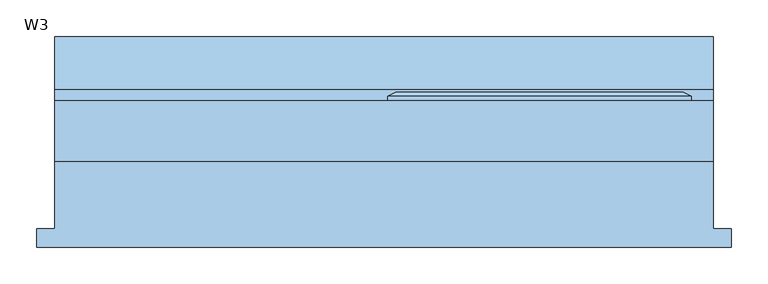
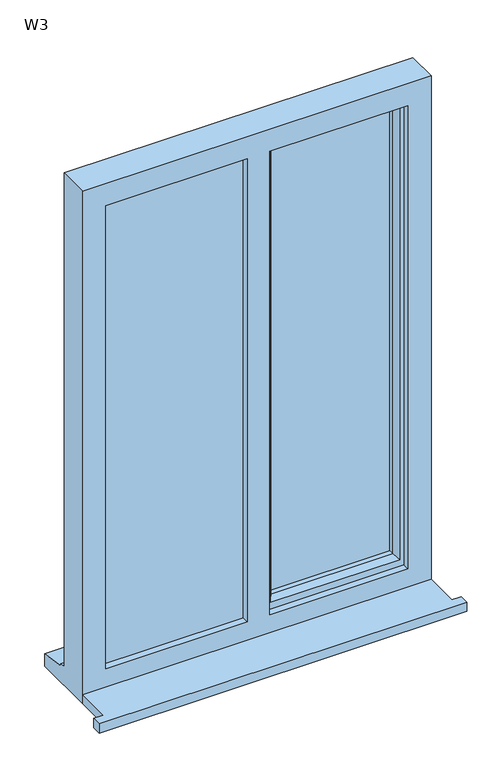
"""IFC4 building model written with IfcOpenShell, lengths in millimetres: window geometry, W3."""

from ifc_helpers import new_model, si_unit, frame, origin, place, context, project, spatial, polyline, outline, extrude, faceted_brep, source, transform, mapped, element, save


def w3_c0944c91(model_context):
    return source(origin(), model_context, "Body", "SolidModel", [
        extrude(outline(polyline([(-760.0, -129.0434322), (-760.0, -104.0434322), (-735.0, -104.0434322), (-735.0, -12.0434322), (165.0, -12.0434322), (165.0, -104.0434322), (190.0, -104.0434322), (190.0, -129.0434322), (-760.0, -129.0434322)])), frame((0.0, 0.0, 1000.0), z_axis=(0.0, 0.0, 1.0), x_axis=(1.0, 0.0, 0.0)), (0.0, 0.0, 1.0), 25.0),
        faceted_brep([(-280.0, 70.9565678, 2370.0), (-280.0, 76.7300705, 2370.0), (-280.0, 76.7300705, 1053.0), (-280.0, 70.9565678, 1053.0), (-270.0, 5.9565678, 2360.0), (-270.0, 70.9565678, 2360.0), (-270.0, 70.9565678, 1063.0), (-270.0, 5.9565678, 1063.0), (-230.0, 20.4494677, 2320.0), (-240.1480377, 5.9565678, 2330.1480377), (-240.1480377, 5.9565678, 1092.8519623), (-230.0, 20.4494677, 1103.0), (-230.0, 34.9565678, 2320.0), (-230.0, 34.9565678, 1103.0), (-240.0, 58.9565678, 2330.0), (-240.0, 34.9565678, 2330.0), (-240.0, 34.9565678, 1093.0), (-240.0, 58.9565678, 1093.0), (-230.0, 76.7300705, 2320.0), (-230.0, 58.9565678, 2320.0), (-230.0, 58.9565678, 1103.0), (-230.0, 76.7300705, 1103.0), (-247.4457548, 82.5035732, 2337.4457548), (-247.4457548, 82.5035732, 1085.5542452), (-269.2153903, 82.5035732, 2359.2153903), (-269.2153903, 82.5035732, 1063.7846097), (135.0, 76.7300705, 1053.0), (135.0, 70.9565678, 1053.0), (125.0, 70.9565678, 1063.0), (125.0, 5.9565678, 1063.0), (95.1480377, 5.9565678, 1092.8519623), (85.0, 20.4494677, 1103.0), (85.0, 34.9565678, 1103.0), (95.0, 34.9565678, 1093.0), (95.0, 58.9565678, 1093.0), (85.0, 58.9565678, 1103.0), (85.0, 76.7300705, 1103.0), (102.4457548, 82.5035732, 1085.5542452), (124.2153903, 82.5035732, 1063.7846097), (135.0, 76.7300705, 2370.0), (135.0, 70.9565678, 2370.0), (125.0, 70.9565678, 2360.0), (125.0, 5.9565678, 2360.0), (95.1480377, 5.9565678, 2330.1480377), (85.0, 20.4494677, 2320.0), (85.0, 34.9565678, 2320.0), (95.0, 34.9565678, 2330.0), (95.0, 58.9565678, 2330.0), (85.0, 58.9565678, 2320.0), (85.0, 76.7300705, 2320.0), (102.4457548, 82.5035732, 2337.4457548), (124.2153903, 82.5035732, 2359.2153903)], [[[0, 1, 2, 3]], [[4, 5, 6, 7]], [[8, 9, 10, 11]], [[12, 8, 11, 13]], [[14, 15, 16, 17]], [[18, 19, 20, 21]], [[22, 18, 21, 23]], [[1, 24, 25, 2]], [[3, 2, 26, 27]], [[7, 6, 28, 29]], [[11, 10, 30, 31]], [[13, 11, 31, 32]], [[17, 16, 33, 34]], [[21, 20, 35, 36]], [[23, 21, 36, 37]], [[2, 25, 38, 26]], [[27, 26, 39, 40]], [[29, 28, 41, 42]], [[31, 30, 43, 44]], [[32, 31, 44, 45]], [[34, 33, 46, 47]], [[36, 35, 48, 49]], [[37, 36, 49, 50]], [[26, 38, 51, 39]], [[40, 39, 1, 0]], [[3, 27, 40, 0], [5, 41, 28, 6]], [[42, 41, 5, 4]], [[7, 29, 42, 4], [9, 43, 30, 10]], [[44, 43, 9, 8]], [[45, 44, 8, 12]], [[15, 46, 33, 16], [13, 32, 45, 12]], [[47, 46, 15, 14]], [[17, 34, 47, 14], [19, 48, 35, 20]], [[49, 48, 19, 18]], [[50, 49, 18, 22]], [[24, 51, 38, 25], [23, 37, 50, 22]], [[39, 51, 24, 1]]]),
        extrude(outline(polyline([(2340.0, -310.0), (2360.0, -310.0), (2360.0, -695.0), (1063.0, -695.0), (1063.0, -310.0), (1083.0, -310.0), (1083.0, -675.0), (2340.0, -675.0), (2340.0, -310.0)])), frame((0.0, 29.9565678, 0.0), z_axis=(0.0, 1.0, 0.0), x_axis=(0.0, 0.0, 1.0)), (0.0, 0.0, 1.0), 41.0),
        faceted_brep([(165.0, -12.0434322, 2400.0), (-735.0, -12.0434322, 2400.0), (-735.0, -12.0434322, 1000.0), (165.0, -12.0434322, 1000.0), (105.0, -12.0434322, 2340.0), (105.0, -12.0434322, 1075.0), (-252.0, -12.0434322, 1075.0), (-252.0, -12.0434322, 2340.0), (-310.0, -12.0434322, 2340.0), (-310.0, -12.0434322, 1075.0), (-675.0, -12.0434322, 1075.0), (-675.0, -12.0434322, 2340.0), (-735.0, 70.9565678, 2400.0), (-735.0, 70.9565678, 1051.0), (-735.0, 85.9565678, 1049.68767), (-735.0, 85.9565678, 1044.7449676), (-735.0, 158.4565678, 1033.8088847), (-735.0, 158.4565678, 1000.0), (165.0, 70.9565678, 2400.0), (165.0, 70.9565678, 1051.0), (-695.0, 70.9565678, 2360.0), (-695.0, 70.9565678, 1063.0), (-310.0, 70.9565678, 1063.0), (-310.0, 70.9565678, 2360.0), (-270.0, 70.9565678, 2360.0), (-270.0, 70.9565678, 1063.0), (125.0, 70.9565678, 1063.0), (125.0, 70.9565678, 2360.0), (-695.0, 5.9565678, 2360.0), (-695.0, 5.9565678, 1063.0), (-300.0, 5.9565678, 2360.0), (-300.0, 5.9565678, 1063.0), (-310.0, 5.9565678, 2340.0), (-675.0, 5.9565678, 2340.0), (-675.0, 5.9565678, 1075.0), (-310.0, 5.9565678, 1075.0), (-270.0, 5.9565678, 2360.0), (125.0, 5.9565678, 2360.0), (125.0, 5.9565678, 1063.0), (-270.0, 5.9565678, 1063.0), (105.0, 5.9565678, 2340.0), (-252.0, 5.9565678, 2340.0), (-252.0, 5.9565678, 1075.0), (105.0, 5.9565678, 1075.0), (-310.0, 29.9565678, 2360.0), (-300.0, 29.9565678, 2360.0), (165.0, 158.4565678, 1000.0), (165.0, 158.4565678, 1033.8088847), (165.0, 85.9565678, 1044.7449676), (165.0, 85.9565678, 1049.68767), (-300.0, 29.9565678, 1063.0), (-310.0, 29.9565678, 1063.0)], [[[0, 1, 2, 3], [4, 5, 6, 7], [8, 9, 10, 11]], [[2, 1, 12, 13, 14, 15, 16, 17]], [[13, 12, 18, 19], [20, 21, 22, 23], [24, 25, 26, 27]], [[21, 20, 28, 29]], [[28, 30, 31, 29], [32, 33, 34, 35]], [[36, 37, 38, 39], [40, 41, 42, 43]], [[33, 11, 10, 34]], [[1, 0, 18, 12]], [[28, 20, 23, 44, 45, 30]], [[27, 37, 36, 24]], [[11, 33, 32, 8]], [[40, 4, 7, 41]], [[19, 18, 0, 3, 46, 47, 48, 49]], [[27, 26, 38, 37]], [[4, 40, 43, 5]], [[45, 50, 31, 30]], [[50, 45, 44, 51]], [[51, 44, 23, 22]], [[25, 24, 36, 39]], [[41, 7, 6, 42]], [[8, 32, 35, 9]], [[46, 3, 2, 17]], [[47, 46, 17, 16]], [[48, 47, 16, 15]], [[49, 48, 15, 14]], [[19, 49, 14, 13]], [[22, 21, 29, 31, 50, 51]], [[26, 25, 39, 38]], [[6, 5, 43, 42]], [[35, 34, 10, 9]]]),
        extrude(outline(polyline([(-695.0, 29.9565678), (-300.0, 29.9565678), (-300.0, 5.9565678), (-695.0, 5.9565678), (-695.0, 29.9565678)])), frame((0.0, 0.0, 1063.0), z_axis=(0.0, 0.0, 1.0), x_axis=(1.0, 0.0, 0.0)), (0.0, 0.0, 1.0), 1297.0),
        extrude(outline(polyline([(95.0, 34.9565678), (-240.0, 34.9565678), (-240.0, 58.9565678), (95.0, 58.9565678), (95.0, 34.9565678)])), frame((0.0, 0.0, 1093.0), z_axis=(0.0, 0.0, 1.0), x_axis=(1.0, 0.0, 0.0)), (0.0, 0.0, 1.0), 1237.0),
    ])


if __name__ == "__main__":
    model = new_model("IFC4")
    model_context = context("Model", 3, world=origin())
    ifc_project = project(units=[si_unit("LENGTHUNIT", "METRE", prefix="MILLI")], contexts=[model_context])
    site = spatial("IfcSite", under=ifc_project)
    building = spatial("IfcBuilding", under=site)
    placement = place(None, origin())
    w3_shape = w3_c0944c91(model_context)
    element("IfcWindow", 1, ObjectType="W3", at=placement, inside=building, context=model_context, shape_type="MappedRepresentation", body=[
        mapped(w3_shape, transform((0.0, 0.0, 0.0), x_axis=(1.0, 0.0, 0.0), y_axis=(0.0, 1.0, 0.0), z_axis=(0.0, 0.0, 1.0))),
    ])
    save(model, "model.ifc")

# Revit data of these elements
# Type "W3"
#   Type Mark = "41"
#   Operation = "DoublePanelVertical"
#   Manufacturer = "Revit"
#   Wrap Layers (Ext) from Ext = 102.5 mm
#   Wrap Layers (Int) from Ext = 177.5 mm
#   Window Board Projection = 25 mm
#   Window Board Extension = 25 mm
#   Rough Width = 900 mm
#   Rough Height = 1400 mm
#   Height = 1400 mm
#   Width = 900 mm
#   Glazing Thickness = 24 mm
#   FrameOffset - External = 50 mm
#   Frame Depth = 65 mm
#   Default Head Height = 2400 mm
#   Cill Depth = 87.5 mm
#   Cavity Closer Width = 50 mm
#   Cavity Closer Offset from Ext = 102.5 mm
#   Cavity Closer Depth = 85 mm
#   Vis - Cavity Closers = yes
#   Material Trim = Window Frame
#   Material Glass = Glass
#   Material Frame = Window Frame
#   Wall Closure = (empty or 0)
# Element 1 (IfcWindow, "W3")
#   Materials on its faces: "Window Frame", "Glass"
# Materials
#   "Window Frame": colour RGB 249 249 249, transparency 0
#   "Glass": class "Glass", colour RGB 245 245 243, transparency 1, Description = "Soda Lime Glass", Cost = 0
